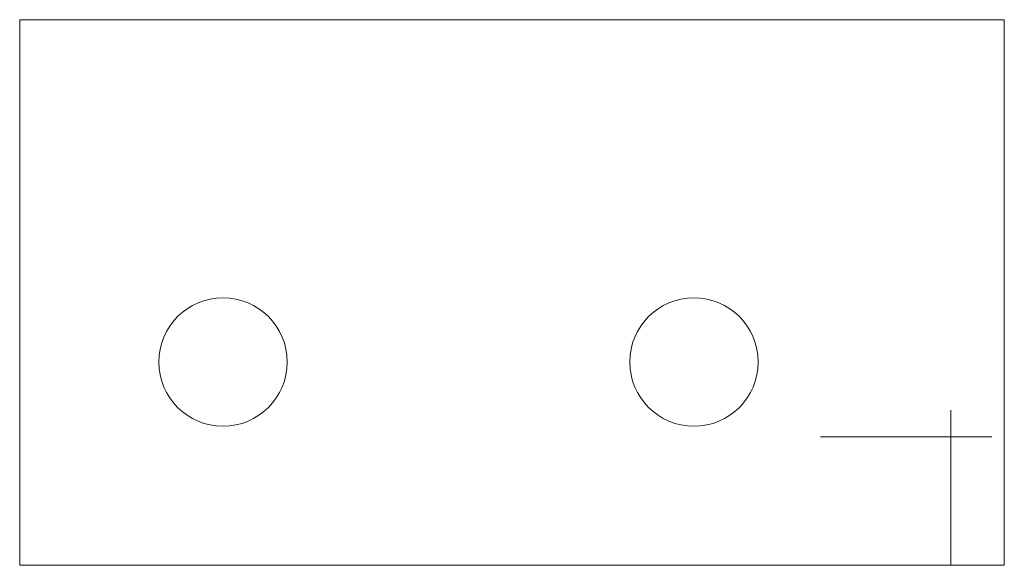
# Model space of a CAD drawing. Units: millimetres. Extents: x 4577.2 to 4669.2, y -26.1 to 24.9.
import ezdxf

# ---------------------------------------------------------------- set-up
doc = ezdxf.new("R2010")
doc.units = ezdxf.units.MM
doc.layers.add('M-CONS', color=8, linetype='Continuous', lineweight=18)

msp = doc.modelspace()

# ---------------------------------------------------------------- linework, layer by layer
at = {"layer": 'M-CONS'}
for p, q in [((4577.19, 24.903), (4577.19, -26.097)), ((4669.19, 24.903), (4577.19, 24.903)), ((4669.19, -26.097), (4669.19, 24.903)), ((4664.19, -26.097, 12), (4664.19, -11.597, 12)), ((4577.19, -26.097), (4669.19, -26.097)), ((4577.19, -26.097), (4596.19, -26.097)), ((4669.19, -26.097), (4664.19, -26.097))]:
    msp.add_line(p, q, dxfattribs=at)
for centre in [(4596.19, -7.097), (4640.19, -7.097)]:
    msp.add_circle(centre, 6, dxfattribs=at)
at = {"layer": 'M-CONS', "extrusion": (0, -1, 0)}
msp.add_circle((4660.027, 112.981, 14.097), 8, dxfattribs=at)

doc.saveas('drawing.dxf')
